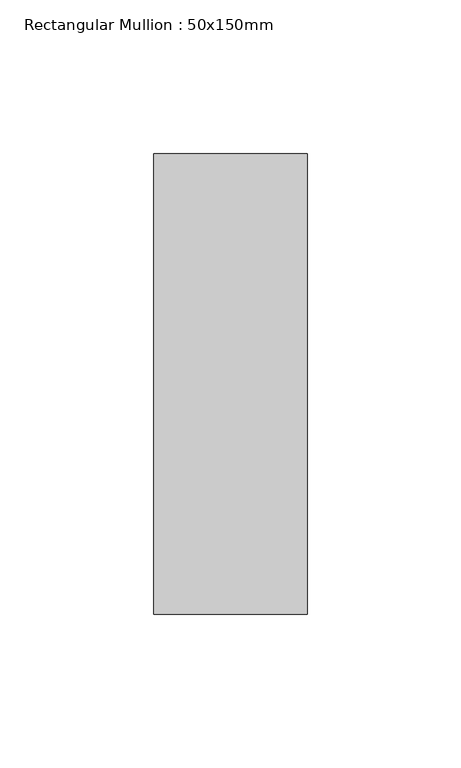
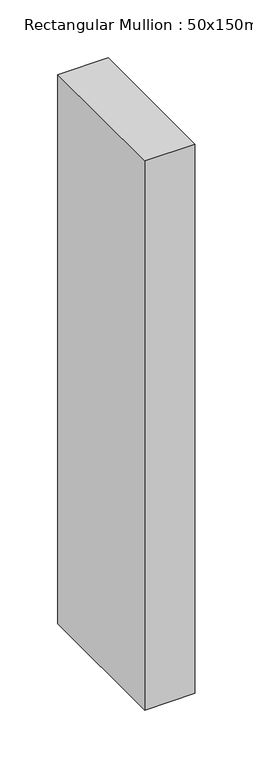
"""IFC4 building model written with IfcOpenShell, lengths in millimetres: member geometry, Rectangular Mullion : 50x150mm."""

from ifc_helpers import new_model, si_unit, frame, origin, place, context, project, spatial, polyline, outline, extrude, source, transform, mapped, element, save


def rectangular_mullion_50x150mm_6d544d31(model_context):
    return source(origin(), model_context, "Body", "SweptSolid", [
        extrude(outline(polyline([(0.0, 75.0), (0.0, -75.0), (-50.0, -75.0), (-50.0, 75.0), (0.0, 75.0)])), frame((0.0, 0.0, -578.65), z_axis=(0.0, 0.0, 1.0), x_axis=(1.0, 0.0, 0.0)), (0.0, 0.0, 1.0), 578.65),
    ])


if __name__ == "__main__":
    model = new_model("IFC4")
    model_context = context("Model", 3, world=origin())
    ifc_project = project(units=[si_unit("LENGTHUNIT", "METRE", prefix="MILLI")], contexts=[model_context])
    site = spatial("IfcSite", under=ifc_project)
    building = spatial("IfcBuilding", under=site)
    placement = place(None, origin())
    rectangular_mullion_50x150mm_shape = rectangular_mullion_50x150mm_6d544d31(model_context)
    element("IfcMember", 1, ObjectType="Rectangular Mullion : 50x150mm", at=placement, inside=building, context=model_context, shape_type="MappedRepresentation", body=[
        mapped(rectangular_mullion_50x150mm_shape, transform((0.0, 0.0, 0.0), x_axis=(1.0, 0.0, 0.0), y_axis=(0.0, 1.0, 0.0), z_axis=(0.0, 0.0, 1.0))),
    ])
    save(model, "model.ifc")

# Revit data of these elements
# Type "Rectangular Mullion : 50x150mm"
#   Keynote = "H11"
#   built-in parameter 1007304 = 0.492126 (stored number, unit not read)
#   built-in parameter 1007301 = 0.082021 (stored number, unit not read)
#   built-in parameter 1007300 = 0.082021 (stored number, unit not read)
# Element 1 (IfcMember, "Rectangular Mullion : 50x150mm")
#   Materials on its faces: "Aluminium"
# Materials
#   "Aluminium": class "Metal", colour RGB 247 247 247, transparency 0, Description = "Aluminium 6061", Cost = 0
